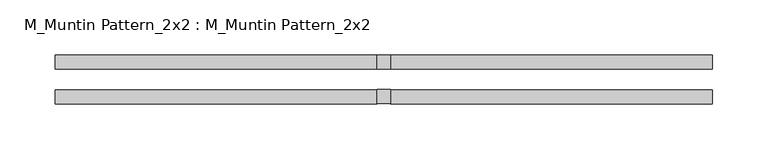
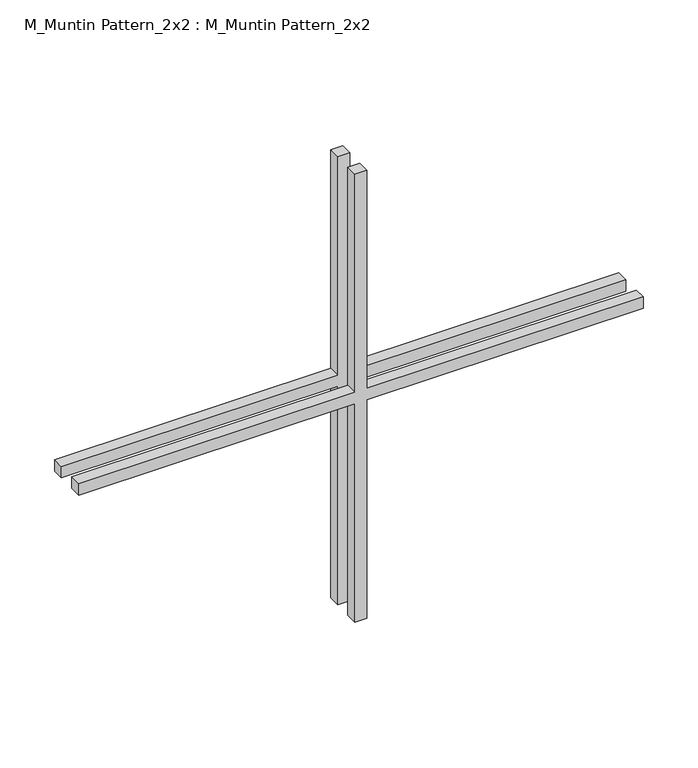
"""IFC4 building model written with IfcOpenShell, lengths in millimetres: proxy geometry, M_Muntin Pattern_2x2 : M_Muntin Pattern_2x2."""

from ifc_helpers import new_model, si_unit, frame, origin, place, context, project, spatial, polyline, outline, extrude, source, transform, mapped, element, save


def m_muntin_pattern_2x2_m_muntin_pattern_2x2_aaec3afb(model_context):
    return source(origin(), model_context, "Body", "SweptSolid", [
        extrude(outline(polyline([(257.1375, -6.35), (257.1375, -298.8), (244.4375, -298.8), (244.4375, -6.35), (0.0, -6.35), (0.0, 6.35), (244.4375, 6.35), (244.4375, 298.8), (257.1375, 298.8), (257.1375, 6.35), (501.575, 6.35), (501.575, -6.35), (257.1375, -6.35)])), frame((0.0, 9.525, 0.0), z_axis=(0.0, 1.0, 0.0), x_axis=(0.0, 0.0, 1.0)), (0.0, 0.0, 1.0), 12.7),
        extrude(outline(polyline([(257.1375, -6.35), (257.1375, -298.8), (244.4375, -298.8), (244.4375, -6.35), (0.0, -6.35), (0.0, 6.35), (244.4375, 6.35), (244.4375, 298.8), (257.1375, 298.8), (257.1375, 6.35), (501.575, 6.35), (501.575, -6.35), (257.1375, -6.35)])), frame((0.0, -22.225, 0.0), z_axis=(0.0, 1.0, 0.0), x_axis=(0.0, 0.0, 1.0)), (0.0, 0.0, 1.0), 12.7),
    ])


if __name__ == "__main__":
    model = new_model("IFC4")
    model_context = context("Model", 3, world=origin())
    ifc_project = project(units=[si_unit("LENGTHUNIT", "METRE", prefix="MILLI")], contexts=[model_context])
    site = spatial("IfcSite", under=ifc_project)
    building = spatial("IfcBuilding", under=site)
    placement = place(None, origin())
    m_muntin_pattern_2x2_m_muntin_pattern_2x2_shape = m_muntin_pattern_2x2_m_muntin_pattern_2x2_aaec3afb(model_context)
    element("IfcBuildingElementProxy", 1, Name="M_Muntin Pattern_2x2 : M_Muntin Pattern_2x2", ObjectType="M_Muntin Pattern_2x2 : M_Muntin Pattern_2x2", at=placement, inside=building, context=model_context, shape_type="MappedRepresentation", body=[
        mapped(m_muntin_pattern_2x2_m_muntin_pattern_2x2_shape, transform((0.0, 0.0, 0.0), x_axis=(1.0, 0.0, 0.0), y_axis=(0.0, 1.0, 0.0), z_axis=(0.0, 0.0, 1.0))),
    ])
    save(model, "model.ifc")

# Revit data of these elements
# Type "M_Muntin Pattern_2x2 : M_Muntin Pattern_2x2"
#   Width [instance default] = 1.2 m
#   Thickness = 0.0127 m
#   Height [instance default] = 1.2 m
#   Distance = 0.01905 m
#   Interior Material [instance default] = none
#   Exterior Material [instance default] = none
#   Default Elevation = 0
# Element 1 (IfcBuildingElementProxy, "M_Muntin Pattern_2x2 : M_Muntin Pattern_2x2")
#   Width = 0.5976 m
#   Height = 0.501575 m
#   Interior Material = Wood - Stained
#   Exterior Material = Clad - White
#   Materials on its faces: "Clad - White", "Wood - Stained"
# Materials
#   "Clad - White": class "Wood", colour RGB 242 242 238, transparency 0, Cost = 0
#   "Wood - Stained": class "Wood", colour RGB 224 178 126, transparency 0, Cost = 0
